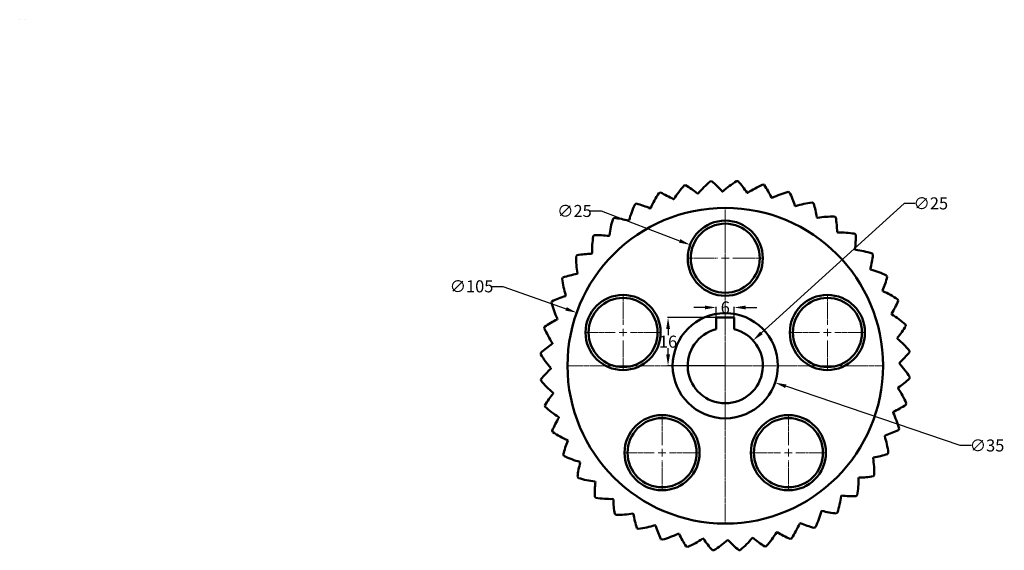
# Model space of a CAD drawing. Units: millimetres. Extents: x 506 to 834, y 506 to 683.
import ezdxf

# ---------------------------------------------------------------- set-up
doc = ezdxf.new("R2010")
doc.units = ezdxf.units.MM
doc.header["$MEASUREMENT"] = 0
doc.linetypes.add('CENTER2', pattern=[1.125, 0.75, -0.125, 0.125, -0.125])
for name, color, linetype, lineweight in [('M-CNTR', 4, 'CENTER2', 18), ('M-DIMS', 2, 'Continuous', 25), ('M-OUTL', 7, 'Continuous', 50)]:
    doc.layers.add(name, color=color, linetype=linetype, lineweight=lineweight)
doc.styles.get("Standard").update_dxf_attribs({"font": 'arial.ttf'})
doc.dimstyles.get("Standard").update_dxf_attribs({"dimtxt": 4, "dimasz": 3.75, "dimexe": 0.18, "dimexo": 0.0625, "dimgap": 0.09, "dimtad": 0, "dimtih": 1, "dimtoh": 1, "dimdec": 0, "dimzin": 0, "dimdsep": 46, "dimtxsty": 'Standard', "dimcen": 0.09, "dimadec": 0, "dimazin": 0, "dimtfac": 1, "dimtdec": 0, "dimtofl": 0, "dimtmove": 0, "dimatfit": 3, "dimfxl": 1, "dimtolj": 1, "dimtzin": 0, "dimarcsym": 0})

# ---------------------------------------------------------------- blocks, each defined once
blk = doc.blocks.new('*U1')
for radius in [12.5, 11.5]:
    blk.add_circle((0, 0), radius)
blk = doc.blocks.new('*U2')
at = {"layer": 'M-OUTL', "color": 0, "linetype": 'ByBlock', "lineweight": -2, "transparency": 16777216}
blk.add_blockref('*U1', (740.72, 603.54), dxfattribs=at)
for p, rotation in [((706.72, 578.84), 72), ((774.72, 578.84), 288), ((719.7, 538.86), 144), ((761.73, 538.86), 216)]:
    blk.add_blockref('*U1', p, dxfattribs=dict(at, rotation=rotation))
blk = doc.blocks.new('*D3')
at = {"layer": 'Defpoints', "color": 0, "transparency": 16777216}
for p in [(729.04, 607.99), (752.4, 599.09)]:
    blk.add_point(p, dxfattribs=at)
at = {"layer": 'M-DIMS', "color": 0, "lineweight": -2, "transparency": 16777216}
for p, q in [((695.68, 619.25), (699.43, 619.25)), ((699.43, 619.25), (725.53, 609.32)), ((740.63, 603.54), (740.81, 603.54)), ((740.72, 603.45), (740.72, 603.63))]:
    blk.add_line(p, q, dxfattribs=at)
at = {"layer": 'M-DIMS', "color": 0, "transparency": 16777216}
blk.add_solid([(725.75, 609.9), (725.31, 608.73), (729.04, 607.99)], dxfattribs=at)
at = {"layer": 'M-DIMS', "color": 0, "transparency": 16777216, "insert": (690.53, 619.25), "char_height": 4, "attachment_point": 5}
blk.add_mtext('\\A1;∅25', dxfattribs=at)
blk = doc.blocks.new('*D4')
at = {"layer": 'Defpoints', "color": 0, "transparency": 16777216}
for p in [(691.27, 585.43), (790.16, 550.14)]:
    blk.add_point(p, dxfattribs=at)
at = {"layer": 'M-DIMS', "color": 0, "lineweight": -2, "transparency": 16777216}
for p, q in [((662.98, 594.19), (666.73, 594.19)), ((666.73, 594.19), (687.74, 586.69)), ((740.63, 567.79), (740.81, 567.79)), ((740.72, 567.7), (740.72, 567.88))]:
    blk.add_line(p, q, dxfattribs=at)
at = {"layer": 'M-DIMS', "color": 0, "transparency": 16777216}
blk.add_solid([(687.95, 587.28), (687.53, 586.11), (691.27, 585.43)], dxfattribs=at)
at = {"layer": 'M-DIMS', "color": 0, "transparency": 16777216, "insert": (656.28, 594.19), "char_height": 4, "attachment_point": 5}
blk.add_mtext('\\A1;∅105', dxfattribs=at)
blk = doc.blocks.new('*D5')
at = {"layer": 'Defpoints', "color": 0, "transparency": 16777216}
for p in [(724.15, 573.41), (757.29, 562.17)]:
    blk.add_point(p, dxfattribs=at)
at = {"layer": 'M-DIMS', "color": 0, "lineweight": -2, "transparency": 16777216}
for p, q in [((740.63, 567.79), (740.81, 567.79)), ((740.72, 567.7), (740.72, 567.88)), ((818.93, 541.26), (760.84, 560.96)), ((822.68, 541.26), (818.93, 541.26))]:
    blk.add_line(p, q, dxfattribs=at)
at = {"layer": 'M-DIMS', "color": 0, "transparency": 16777216}
blk.add_solid([(761.04, 561.55), (760.64, 560.37), (757.29, 562.17)], dxfattribs=at)
at = {"layer": 'M-DIMS', "color": 0, "transparency": 16777216, "insert": (827.83, 541.26), "char_height": 4, "attachment_point": 5}
blk.add_mtext('\\A1;∅35', dxfattribs=at)
blk = doc.blocks.new('*D6')
at = {"layer": 'Defpoints', "color": 0, "transparency": 16777216}
for p in [(749.98, 576.19), (731.46, 559.39)]:
    blk.add_point(p, dxfattribs=at)
at = {"layer": 'M-DIMS', "color": 0, "lineweight": -2, "transparency": 16777216}
for p, q in [((800.22, 621.78), (752.75, 578.71)), ((803.97, 621.78), (800.22, 621.78)), ((740.63, 567.79), (740.81, 567.79)), ((740.72, 567.7), (740.72, 567.88))]:
    blk.add_line(p, q, dxfattribs=at)
at = {"layer": 'M-DIMS', "color": 0, "transparency": 16777216}
blk.add_solid([(752.33, 579.17), (753.17, 578.25), (749.98, 576.19)], dxfattribs=at)
at = {"layer": 'M-DIMS', "color": 0, "transparency": 16777216, "insert": (809.12, 621.78), "char_height": 4, "attachment_point": 5}
blk.add_mtext('\\A1;∅25', dxfattribs=at)
blk = doc.blocks.new('*D7')
at = {"layer": 'Defpoints', "color": 0, "transparency": 16777216}
for p in [(721.69, 583.79), (740.81, 583.79), (740.81, 567.79)]:
    blk.add_point(p, dxfattribs=at)
at = {"layer": 'M-DIMS', "color": 0, "lineweight": -2, "transparency": 16777216}
for p, q in [((740.75, 583.79), (721.51, 583.79)), ((721.69, 580.04), (721.69, 577.92)), ((721.69, 571.54), (721.69, 573.66)), ((740.75, 567.79), (721.51, 567.79))]:
    blk.add_line(p, q, dxfattribs=at)
at = {"layer": 'M-DIMS', "color": 0, "transparency": 16777216}
for points in [[(721.07, 580.04), (722.32, 580.04), (721.69, 583.79)], [(721.07, 571.54), (722.32, 571.54), (721.69, 567.79)]]:
    blk.add_solid(points, dxfattribs=at)
at = {"layer": 'M-DIMS', "color": 0, "transparency": 16777216, "insert": (721.69, 575.79), "char_height": 4, "attachment_point": 5}
blk.add_mtext('\\A1;16', dxfattribs=at)
blk = doc.blocks.new('*D8')
at = {"layer": 'Defpoints', "color": 0, "transparency": 16777216}
for p in [(743.72, 587.16), (737.72, 583.79), (743.72, 583.79)]:
    blk.add_point(p, dxfattribs=at)
at = {"layer": 'M-DIMS', "color": 0, "lineweight": -2, "transparency": 16777216}
for p, q in [((733.97, 587.16), (730.22, 587.16)), ((737.72, 583.85), (737.72, 587.34)), ((743.72, 583.85), (743.72, 587.34)), ((747.47, 587.16), (751.22, 587.16))]:
    blk.add_line(p, q, dxfattribs=at)
at = {"layer": 'M-DIMS', "color": 0, "transparency": 16777216}
for points in [[(733.97, 587.78), (733.97, 586.53), (737.72, 587.16)], [(747.47, 587.78), (747.47, 586.53), (743.72, 587.16)]]:
    blk.add_solid(points, dxfattribs=at)
at = {"layer": 'M-DIMS', "color": 0, "transparency": 16777216, "insert": (740.72, 587.16), "char_height": 4, "attachment_point": 5}
blk.add_mtext('\\A1;6', dxfattribs=at)
blk = doc.blocks.new('*U9')
at = {"layer": 'M-CNTR', "color": 0, "transparency": 16777216}
for p, q in [((0, 2.5), (0, 12.62)), ((-12.62, 0), (-2.5, 0)), ((2.5, 0), (12.62, 0)), ((0, -12.62), (0, -2.5))]:
    blk.add_line(p, q, dxfattribs=at)
at = {"layer": 'M-CNTR', "color": 0, "linetype": 'Continuous', "transparency": 16777216}
for p, q in [((-1.25, 0), (1.25, 0)), ((0, -1.25), (0, 1.25))]:
    blk.add_line(p, q, dxfattribs=at)
blk = doc.blocks.new('*U10')
at = {"layer": 'M-CNTR', "color": 0, "transparency": 16777216}
for p, q in [((0, 2.5), (0, 12.62)), ((-12.62, 0), (-2.5, 0)), ((2.5, 0), (12.62, 0)), ((0, -12.62), (0, -2.5))]:
    blk.add_line(p, q, dxfattribs=at)
at = {"layer": 'M-CNTR', "color": 0, "linetype": 'Continuous', "transparency": 16777216}
for p, q in [((-1.25, 0), (1.25, 0)), ((0, -1.25), (0, 1.25))]:
    blk.add_line(p, q, dxfattribs=at)
blk = doc.blocks.new('*U11')
at = {"layer": 'M-CNTR', "color": 0, "transparency": 16777216}
for p, q in [((0, 2.5), (0, 12.62)), ((-12.62, 0), (-2.5, 0)), ((2.5, 0), (12.62, 0)), ((0, -12.62), (0, -2.5))]:
    blk.add_line(p, q, dxfattribs=at)
at = {"layer": 'M-CNTR', "color": 0, "linetype": 'Continuous', "transparency": 16777216}
for p, q in [((-1.25, 0), (1.25, 0)), ((0, -1.25), (0, 1.25))]:
    blk.add_line(p, q, dxfattribs=at)
blk = doc.blocks.new('*U12')
at = {"layer": 'M-CNTR', "color": 0, "transparency": 16777216}
for p, q in [((0, 2.5), (0, 12.62)), ((-12.62, 0), (-2.5, 0)), ((2.5, 0), (12.62, 0)), ((0, -12.62), (0, -2.5))]:
    blk.add_line(p, q, dxfattribs=at)
at = {"layer": 'M-CNTR', "color": 0, "linetype": 'Continuous', "transparency": 16777216}
for p, q in [((-1.25, 0), (1.25, 0)), ((0, -1.25), (0, 1.25))]:
    blk.add_line(p, q, dxfattribs=at)
blk = doc.blocks.new('*U13')
at = {"layer": 'M-CNTR', "color": 0, "transparency": 16777216}
for p, q in [((0, 2.5), (0, 12.62)), ((-12.62, 0), (-2.5, 0)), ((2.5, 0), (12.62, 0)), ((0, -12.62), (0, -2.5))]:
    blk.add_line(p, q, dxfattribs=at)
at = {"layer": 'M-CNTR', "color": 0, "linetype": 'Continuous', "transparency": 16777216}
for p, q in [((-1.25, 0), (1.25, 0)), ((0, -1.25), (0, 1.25))]:
    blk.add_line(p, q, dxfattribs=at)
blk = doc.blocks.new('*U14')
at = {"layer": 'M-CNTR', "color": 0, "transparency": 16777216}
for p, q in [((0, 3.5), (0, 17.62)), ((-17.62, 0), (-3.5, 0)), ((3.5, 0), (17.62, 0)), ((0, -17.62), (0, -3.5))]:
    blk.add_line(p, q, dxfattribs=at)
at = {"layer": 'M-CNTR', "color": 0, "linetype": 'Continuous', "transparency": 16777216}
for p, q in [((-1.75, 0), (1.75, 0)), ((0, -1.75), (0, 1.75))]:
    blk.add_line(p, q, dxfattribs=at)
blk = doc.blocks.new('*U15')
at = {"layer": 'M-CNTR', "color": 0, "transparency": 16777216}
for p, q in [((0, 10.5), (0, 52.62)), ((-52.62, 0), (-10.5, 0)), ((10.5, 0), (52.62, 0)), ((0, -52.62), (0, -10.5))]:
    blk.add_line(p, q, dxfattribs=at)
at = {"layer": 'M-CNTR', "color": 0, "linetype": 'Continuous', "transparency": 16777216}
for p, q in [((0, -5.25), (0, 5.25)), ((-5.25, 0), (5.25, 0))]:
    blk.add_line(p, q, dxfattribs=at)

msp = doc.modelspace()

# ---------------------------------------------------------------- linework, layer by layer
at = {"layer": 'M-OUTL'}
for p, q in [((505.93, 682.86), (505.93, 682.86)), ((507.93, 682.86), (507.93, 682.86)), ((735.72, 629.08), (736.22, 629.12)), ((744.49, 629.17), (744.99, 629.14)), ((727.05, 627.75), (727.54, 627.86)), ((753.19, 628.01), (753.68, 627.91)), ((718.65, 625.19), (719.12, 625.37)), ((723.42, 623.15), (723.66, 623.22)), ((731.48, 625.05), (731.72, 625.09)), ((739.72, 625.78), (739.97, 625.78)), ((747.98, 625.33), (748.23, 625.3)), ((756.1, 623.71), (756.33, 623.65)), ((761.63, 625.62), (762.11, 625.45)), ((710.71, 621.47), (711.15, 621.71)), ((715.72, 620.12), (715.94, 620.23)), ((763.9, 620.95), (764.13, 620.86)), ((769.65, 622.06), (770.09, 621.82)), ((703.37, 616.65), (703.77, 616.95)), ((708.53, 616.03), (708.73, 616.17)), ((771.23, 617.11), (771.44, 616.98)), ((777.08, 617.39), (777.48, 617.09)), ((696.8, 610.84), (697.15, 611.2)), ((701.99, 610.96), (702.17, 611.12)), ((777.94, 612.27), (778.13, 612.11)), ((783.77, 611.71), (784.13, 611.35)), ((783.89, 606.52), (784.06, 606.34)), ((691.12, 604.15), (691.42, 604.55)), ((696.24, 605.01), (696.4, 605.2)), ((789.58, 605.13), (789.88, 604.73)), ((788.96, 599.98), (789.1, 599.78)), ((686.45, 596.72), (686.69, 597.16)), ((691.39, 598.3), (691.52, 598.51)), ((794.4, 597.8), (794.64, 597.36)), ((687.55, 590.97), (687.65, 591.19)), ((793.05, 592.79), (793.16, 592.57)), ((798.12, 589.85), (798.3, 589.39)), ((682.89, 588.7), (683.06, 589.17)), ((684.8, 583.17), (684.86, 583.4)), ((737.72, 583.79), (743.72, 583.79)), ((737.72, 579.92), (737.72, 583.79)), ((743.72, 579.92), (743.72, 583.79)), ((796.08, 585.09), (796.15, 584.85)), ((680.5, 580.26), (680.6, 580.75)), ((800.68, 581.46), (800.79, 580.97)), ((797.98, 577.03), (798.02, 576.79)), ((683.18, 575.05), (683.21, 575.3)), ((679.34, 571.56), (679.37, 572.06)), ((802.02, 572.79), (802.05, 572.29)), ((682.73, 566.79), (682.72, 567.03)), ((798.71, 568.79), (798.71, 568.54)), ((802.1, 564.01), (802.07, 563.51)), ((679.42, 562.79), (679.38, 563.29)), ((798.26, 560.52), (798.23, 560.28)), ((683.46, 558.55), (683.42, 558.79)), ((680.76, 554.12), (680.65, 554.6)), ((800.94, 555.32), (800.84, 554.83)), ((685.36, 550.49), (685.29, 550.73)), ((796.64, 552.41), (796.58, 552.17)), ((683.31, 545.72), (683.14, 546.19)), ((793.89, 544.61), (793.79, 544.38)), ((798.55, 546.87), (798.38, 546.4)), ((688.38, 542.79), (688.28, 543.01)), ((687.04, 537.78), (686.8, 538.22)), ((794.99, 538.85), (794.75, 538.41)), ((692.47, 535.59), (692.34, 535.8)), ((790.05, 537.28), (789.92, 537.07)), ((691.86, 530.44), (691.55, 530.84)), ((790.32, 531.43), (790.02, 531.02)), ((697.55, 529.06), (697.38, 529.24)), ((785.2, 530.57), (785.04, 530.38)), ((779.45, 524.62), (779.27, 524.45)), ((784.64, 524.74), (784.29, 524.38)), ((697.67, 523.87), (697.31, 524.22)), ((703.5, 523.31), (703.31, 523.46)), ((704.36, 518.19), (703.95, 518.49)), ((710.21, 518.46), (710, 518.59)), ((772.91, 519.54), (772.71, 519.41)), ((778.06, 518.93), (777.67, 518.62)), ((717.54, 514.62), (717.31, 514.72)), ((765.72, 515.45), (765.5, 515.35)), ((711.79, 513.52), (711.34, 513.76)), ((725.34, 511.86), (725.1, 511.93)), ((758.02, 512.43), (757.78, 512.35)), ((770.73, 514.11), (770.29, 513.86)), ((719.8, 509.95), (719.33, 510.13)), ((733.46, 510.24), (733.21, 510.28)), ((741.72, 509.8), (741.47, 509.79)), ((749.96, 510.53), (749.72, 510.49)), ((762.79, 510.38), (762.32, 510.21)), ((728.25, 507.57), (727.76, 507.67)), ((736.95, 506.4), (736.44, 506.44)), ((745.72, 506.49), (745.22, 506.45)), ((754.39, 507.83), (753.9, 507.72))]:
    msp.add_line(p, q, dxfattribs=at)
for radius in [52.5, 17.5]:
    msp.add_circle((740.72, 567.79), radius, dxfattribs=at)
for centre, radius, start, end in [((715.93, 604.38), 32, 41.9701, 50.6454), ((761.33, 601.96), 32, 121.7404, 131.8808), ((721.39, 607.54), 32, 33.7883, 42.4635), ((750.87, 606.38), 32, 138.104, 148.2445), ((710.97, 600.48), 32, 50.152, 58.8272), ((756.26, 604.54), 32, 129.9222, 140.0626), ((765.98, 598.68), 32, 113.5586, 123.699), ((727.24, 609.88), 32, 25.6065, 34.2817), ((745.27, 607.43), 32, 146.2858, 156.4263), ((706.62, 595.91), 32, 58.3338, 67.009), ((770.12, 594.77), 32, 105.3767, 115.5172), ((733.37, 611.37), 32, 17.4247, 26.0999), ((739.58, 607.68), 32, 154.4676, 164.6081), ((702.97, 590.77), 32, 66.5156, 75.1908), ((773.66, 590.31), 32, 97.1949, 107.3354), ((739.65, 611.97), 32, 9.2429, 17.9181), ((733.92, 607.11), 32, 162.6495, 172.7899), ((700.08, 585.17), 32, 74.6974, 83.3726), ((776.53, 585.39), 32, 89.0131, 99.1536), ((745.95, 611.68), 32, 1.0611, 9.7363), ((728.39, 605.74), 32, 170.8313, 180.9717), ((698.02, 579.21), 32, 82.8792, 91.5545), ((778.67, 580.12), 32, 80.8313, 90.9717), ((752.14, 610.49), 32, 352.8792, 1.5545), ((780.04, 574.59), 32, 72.6495, 82.7899), ((723.12, 603.6), 32, 179.0131, 189.1536), ((696.83, 573.01), 32, 91.0611, 99.7363), ((758.1, 608.43), 32, 344.6974, 353.3726), ((780.61, 568.92), 32, 64.4676, 74.6081), ((718.2, 600.73), 32, 187.1949, 197.3354), ((696.53, 566.71), 32, 99.2429, 107.9181), ((763.71, 605.54), 32, 336.5156, 345.1908), ((697.14, 560.44), 32, 107.4247, 116.0999), ((780.36, 563.24), 32, 56.2858, 66.4263), ((713.74, 597.19), 32, 195.3767, 205.5172), ((768.84, 601.88), 32, 328.3338, 337.009), ((779.31, 557.64), 32, 48.104, 58.2445), ((709.83, 593.05), 32, 203.5586, 213.699), ((698.63, 554.31), 32, 115.6065, 124.2817), ((773.41, 597.54), 32, 320.152, 328.8272), ((740.72, 567.79), 12.5, 103.8865, 76.1135), ((777.47, 552.25), 32, 39.9222, 50.0626), ((700.97, 548.46), 32, 123.7883, 132.4635), ((706.55, 588.4), 32, 211.7404, 221.8808), ((777.31, 592.58), 32, 311.9701, 320.6454), ((774.89, 547.18), 32, 31.7404, 41.8808), ((704.13, 543), 32, 131.9701, 140.6454), ((703.96, 583.32), 32, 219.9222, 230.0626), ((780.47, 587.12), 32, 303.7883, 312.4635), ((708.03, 538.04), 32, 140.152, 148.8272), ((771.61, 542.53), 32, 23.5586, 33.699), ((702.13, 577.94), 32, 228.104, 238.2445), ((782.81, 581.27), 32, 295.6065, 304.2817), ((712.59, 533.69), 32, 148.3338, 157.009), ((767.7, 538.39), 32, 15.3767, 25.5172), ((701.08, 572.34), 32, 236.2858, 246.4263), ((763.24, 534.85), 32, 7.1949, 17.3354), ((784.3, 575.14), 32, 287.4247, 296.0999), ((717.73, 530.04), 32, 156.5156, 165.1908), ((700.83, 566.65), 32, 244.4676, 254.6081), ((784.91, 568.86), 32, 279.2429, 287.9181), ((723.34, 527.15), 32, 164.6974, 173.3726), ((758.32, 531.98), 32, 359.0131, 9.1536), ((784.61, 562.56), 32, 271.0611, 279.7363), ((701.4, 560.99), 32, 252.6495, 262.7899), ((729.3, 525.09), 32, 172.8792, 181.5545), ((753.05, 529.84), 32, 350.8313, 0.9717), ((747.52, 528.47), 32, 342.6495, 352.7899), ((783.42, 556.37), 32, 262.8792, 271.5545), ((702.77, 555.46), 32, 260.8313, 270.9717), ((735.49, 523.9), 32, 181.0611, 189.7363), ((704.91, 550.18), 32, 269.0131, 279.1536), ((741.79, 523.6), 32, 189.2429, 197.9181), ((741.86, 527.9), 32, 334.4676, 344.6081), ((781.36, 550.41), 32, 254.6974, 263.3726), ((707.78, 545.27), 32, 277.1949, 287.3354), ((748.07, 524.2), 32, 197.4247, 206.0999), ((736.17, 528.14), 32, 326.2858, 336.4263), ((778.47, 544.8), 32, 246.5156, 255.1908), ((711.32, 540.81), 32, 285.3767, 295.5172), ((754.2, 525.69), 32, 205.6065, 214.2817), ((730.57, 529.2), 32, 318.104, 328.2445), ((774.82, 539.66), 32, 238.3338, 247.009), ((715.46, 536.9), 32, 293.5586, 303.699), ((760.05, 528.04), 32, 213.7883, 222.4635), ((720.11, 533.62), 32, 301.7404, 311.8808), ((765.51, 531.2), 32, 221.9701, 230.6454), ((725.18, 531.03), 32, 309.9222, 320.0626), ((770.47, 535.1), 32, 230.152, 238.8272)]:
    msp.add_arc(centre, radius, start, end, dxfattribs=at)

# ---------------------------------------------------------------- block references
at = {"layer": 'M-CNTR'}
for name, p in [('*U15', (740.72, 567.79)), ('*U10', (740.72, 603.54)), ('*U9', (706.72, 578.84)), ('*U11', (774.72, 578.84)), ('*U14', (740.72, 567.79)), ('*U13', (719.7, 538.86)), ('*U12', (761.73, 538.86))]:
    msp.add_blockref(name, p, dxfattribs=at)
at = {"layer": 'M-OUTL'}
msp.add_blockref('*U2', (0, 0), dxfattribs=at)

# ---------------------------------------------------------------- dimensions: what is measured, and where the dimension line sits
at = {"layer": 'M-DIMS'}
for p1, p2, picture, middle in [((731.46, 559.39), (749.98, 576.19), '*D6', (809.12, 621.78)), ((752.4, 599.09), (729.04, 607.99), '*D3', (690.53, 619.25)), ((790.16, 550.14), (691.27, 585.43), '*D4', (656.28, 594.19)), ((724.15, 573.41), (757.29, 562.17), '*D5', (827.83, 541.26))]:
    dim = msp.add_diameter_dim_2p(p1=p1, p2=p2, dimstyle='Standard', override={"dimclrd": 0, "dimclre": 0, "dimclrt": 0}, dxfattribs=at)
    dim.commit()
    dim.dimension.update_dxf_attribs({"geometry": picture, "text_midpoint": middle, "dimtype": 163})
dim = msp.add_linear_dim(base=(743.72, 587.16), p1=(737.72, 583.79), p2=(743.72, 583.79), dimstyle='Standard', override={"dimclrd": 0, "dimclre": 0, "dimclrt": 0}, dxfattribs=at)
dim.commit()
dim.dimension.update_dxf_attribs({"geometry": '*D8', "text_midpoint": (740.72, 587.16)})
dim = msp.add_linear_dim(base=(721.69, 583.79), p1=(740.81, 567.79), p2=(740.81, 583.79), angle=90, dimstyle='Standard', override={"dimclrd": 0, "dimclre": 0, "dimclrt": 0}, dxfattribs=at)
dim.commit()
dim.dimension.update_dxf_attribs({"geometry": '*D7', "text_midpoint": (721.69, 575.79)})

doc.saveas('drawing.dxf')
